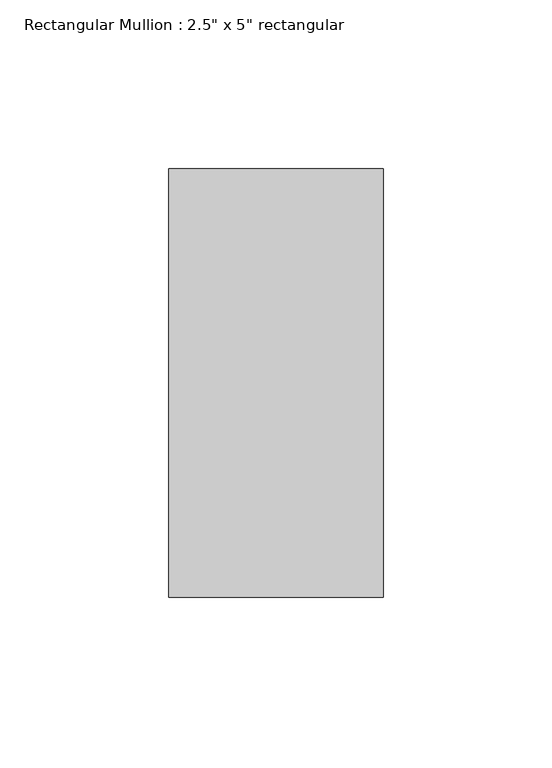
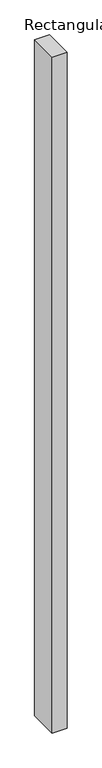
"""IFC4 building model written with IfcOpenShell, lengths in millimetres: member geometry."""

from ifc_helpers import new_model, si_unit, frame, origin, place, context, project, spatial, polyline, outline, extrude, source, transform, mapped, element, save


def member_03093db6(model_context):
    return source(origin(), model_context, "Body", "SweptSolid", [
        extrude(outline(polyline([(31.75, 63.5), (31.75, -63.5), (-31.75, -63.5), (-31.75, 63.5), (31.75, 63.5)])), frame((0.0, 0.0, -3011.3632737), z_axis=(0.0, 0.0, 1.0), x_axis=(1.0, 0.0, 0.0)), (0.0, 0.0, 1.0), 3011.3632737),
    ])


if __name__ == "__main__":
    model = new_model("IFC4")
    model_context = context("Model", 3, world=origin())
    ifc_project = project(units=[si_unit("LENGTHUNIT", "METRE", prefix="MILLI")], contexts=[model_context])
    site = spatial("IfcSite", under=ifc_project)
    building = spatial("IfcBuilding", under=site)
    placement = place(None, origin())
    member_shape = member_03093db6(model_context)
    element("IfcMember", 1, ObjectType="Rectangular Mullion : 2.5\" x 5\" rectangular", at=placement, inside=building, context=model_context, shape_type="MappedRepresentation", body=[
        mapped(member_shape, transform((0.0, 0.0, 0.0), x_axis=(1.0, 0.0, 0.0), y_axis=(0.0, 1.0, 0.0), z_axis=(0.0, 0.0, 1.0))),
    ])
    save(model, "model.ifc")

# Revit data of these elements
# Type "Rectangular Mullion : 2.5\" x 5\" rectangular"
#   built-in parameter 1007304 = 0.416667 (stored number, unit not read)
#   built-in parameter 1007301 = 0.104167 (stored number, unit not read)
#   built-in parameter 1007300 = 0.104167 (stored number, unit not read)
